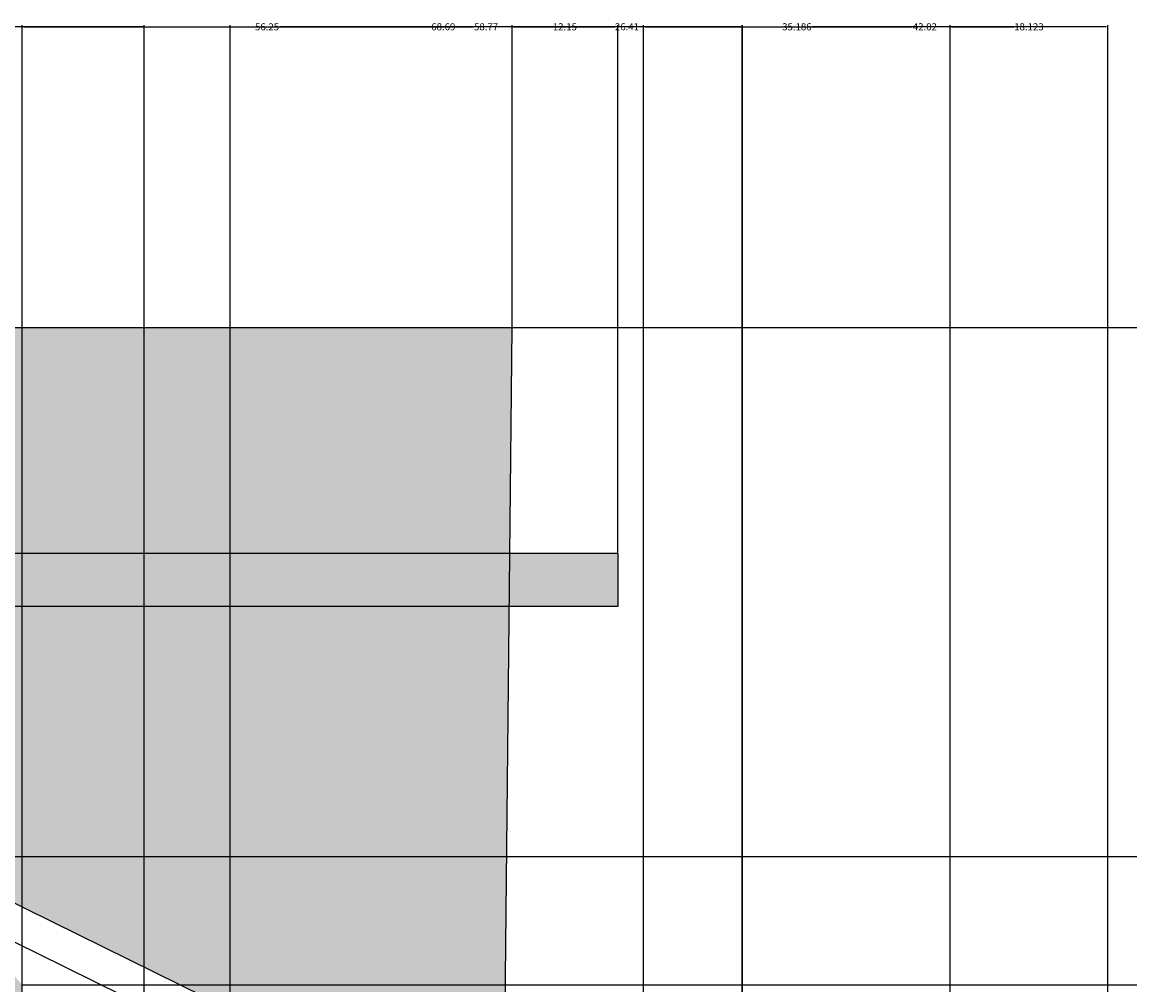
# Model space of a CAD drawing. Units: inches. Extents: x 36 to 594, y 79 to 831.
# Tile 28 of 30: x 342 to 469, y 721 to 831. Entities that reach past the tile are written whole.
import ezdxf

# ---------------------------------------------------------------- set-up
doc = ezdxf.new("R2010")
doc.units = ezdxf.units.IN
doc.header["$MEASUREMENT"] = 0
for name, color, linetype, lineweight in [('A-ANNO-DIMS', 2, 'Continuous', 18), ('A-ELEV', 7, 'Continuous', 25), ('A-ELEV-PATT', 8, 'Continuous', 13)]:
    doc.layers.add(name, color=color, linetype=linetype, lineweight=lineweight)
doc.styles.get("Standard").update_dxf_attribs({"font": 'arial.ttf'})
doc.dimstyles.get("Standard").update_dxf_attribs({"dimtxt": 0.8125, "dimasz": 0.18, "dimexe": 0.18, "dimexo": 0.0625, "dimgap": 0.09, "dimtad": 0, "dimtih": 1, "dimtoh": 1, "dimdec": 4, "dimzin": 0, "dimdsep": 46, "dimlunit": 4, "dimtxsty": 'Standard', "dimcen": 0.09, "dimadec": 0, "dimazin": 0, "dimtfac": 1, "dimtdec": 4, "dimtofl": 0, "dimtmove": 0, "dimatfit": 3, "dimfxl": 1, "dimtolj": 1, "dimtzin": 0, "dimarcsym": 0})

# ---------------------------------------------------------------- blocks, each defined once
blk = doc.blocks.new('*D16')
at = {"layer": 'A-ANNO-DIMS', "color": 0, "lineweight": -2, "transparency": 16777216}
for p, q in [((269.36, 796.11), (269.36, 830.73)), ((341.84, 720.66), (341.84, 830.73)), ((269.54, 830.55), (304.14, 830.55)), ((341.66, 830.55), (307.06, 830.55))]:
    blk.add_line(p, q, dxfattribs=at)
at = {"layer": 'A-ANNO-DIMS', "color": 0, "transparency": 16777216}
for points in [[(269.54, 830.58), (269.54, 830.52), (269.36, 830.55)], [(341.66, 830.58), (341.66, 830.52), (341.84, 830.55)]]:
    blk.add_solid(points, dxfattribs=at)
at = {"layer": 'Defpoints', "color": 0, "transparency": 16777216}
for p in [(341.84, 830.55), (269.36, 796.05), (341.84, 720.59)]:
    blk.add_point(p, dxfattribs=at)
at = {"layer": 'A-ANNO-DIMS', "color": 0, "transparency": 16777216, "insert": (305.6, 830.55), "char_height": 0.812, "attachment_point": 5}
blk.add_mtext('\\A1;72.48', dxfattribs=at)
blk = doc.blocks.new('*D17')
at = {"layer": 'A-ANNO-DIMS', "color": 0, "lineweight": -2, "transparency": 16777216}
for p, q in [((341.84, 720.66), (341.84, 830.73)), ((398.09, 796.11), (398.09, 830.73)), ((342.02, 830.55), (368.5, 830.55)), ((397.91, 830.55), (371.43, 830.55))]:
    blk.add_line(p, q, dxfattribs=at)
at = {"layer": 'A-ANNO-DIMS', "color": 0, "transparency": 16777216}
for points in [[(342.02, 830.58), (342.02, 830.52), (341.84, 830.55)], [(397.91, 830.58), (397.91, 830.52), (398.09, 830.55)]]:
    blk.add_solid(points, dxfattribs=at)
at = {"layer": 'Defpoints', "color": 0, "transparency": 16777216}
for p in [(398.09, 830.55), (398.09, 796.05), (341.84, 720.59)]:
    blk.add_point(p, dxfattribs=at)
at = {"layer": 'A-ANNO-DIMS', "color": 0, "transparency": 16777216, "insert": (369.96, 830.55), "char_height": 0.812, "attachment_point": 5}
blk.add_mtext('\\A1;56.25', dxfattribs=at)
blk = doc.blocks.new('*D18')
at = {"layer": 'A-ANNO-DIMS', "color": 0, "lineweight": -2, "transparency": 16777216}
for p, q in [((398.09, 796.11), (398.09, 830.73)), ((424.5, 594.27), (424.5, 830.73)), ((398.27, 830.55), (409.9, 830.55)), ((424.32, 830.55), (412.68, 830.55))]:
    blk.add_line(p, q, dxfattribs=at)
at = {"layer": 'A-ANNO-DIMS', "color": 0, "transparency": 16777216}
for points in [[(398.27, 830.58), (398.27, 830.52), (398.09, 830.55)], [(424.32, 830.58), (424.32, 830.52), (424.5, 830.55)]]:
    blk.add_solid(points, dxfattribs=at)
at = {"layer": 'Defpoints', "color": 0, "transparency": 16777216}
for p in [(424.5, 830.55), (398.09, 796.05), (424.5, 594.21)]:
    blk.add_point(p, dxfattribs=at)
at = {"layer": 'A-ANNO-DIMS', "color": 0, "transparency": 16777216, "insert": (411.29, 830.55), "char_height": 0.812, "attachment_point": 5}
blk.add_mtext('\\A1;26.41', dxfattribs=at)
blk = doc.blocks.new('*D19')
at = {"layer": 'A-ANNO-DIMS', "color": 0, "lineweight": -2, "transparency": 16777216}
for p, q in [((424.5, 594.27), (424.5, 830.73)), ((466.51, 668.28), (466.51, 830.73)), ((424.68, 830.55), (444.03, 830.55)), ((466.33, 830.55), (446.98, 830.55))]:
    blk.add_line(p, q, dxfattribs=at)
at = {"layer": 'A-ANNO-DIMS', "color": 0, "transparency": 16777216}
for points in [[(424.68, 830.58), (424.68, 830.52), (424.5, 830.55)], [(466.33, 830.58), (466.33, 830.52), (466.51, 830.55)]]:
    blk.add_solid(points, dxfattribs=at)
at = {"layer": 'Defpoints', "color": 0, "transparency": 16777216}
for p in [(466.51, 830.55), (466.51, 668.22), (424.5, 594.21)]:
    blk.add_point(p, dxfattribs=at)
at = {"layer": 'A-ANNO-DIMS', "color": 0, "transparency": 16777216, "insert": (445.5, 830.55), "char_height": 0.812, "attachment_point": 5}
blk.add_mtext('\\A1;42.02', dxfattribs=at)
blk = doc.blocks.new('*D20')
at = {"layer": 'A-ANNO-DIMS', "color": 0, "lineweight": -2, "transparency": 16777216}
for p, q in [((365.73, 594.27), (365.73, 830.73)), ((424.5, 594.27), (424.5, 830.73)), ((365.91, 830.55), (393.65, 830.55)), ((424.32, 830.55), (396.57, 830.55))]:
    blk.add_line(p, q, dxfattribs=at)
at = {"layer": 'A-ANNO-DIMS', "color": 0, "transparency": 16777216}
for points in [[(365.91, 830.58), (365.91, 830.52), (365.73, 830.55)], [(424.32, 830.58), (424.32, 830.52), (424.5, 830.55)]]:
    blk.add_solid(points, dxfattribs=at)
at = {"layer": 'Defpoints', "color": 0, "transparency": 16777216}
for p in [(424.5, 830.55), (365.73, 594.21), (424.5, 594.21)]:
    blk.add_point(p, dxfattribs=at)
at = {"layer": 'A-ANNO-DIMS', "color": 0, "transparency": 16777216, "insert": (395.11, 830.55), "char_height": 0.812, "attachment_point": 5}
blk.add_mtext('\\A1;58.77', dxfattribs=at)
blk = doc.blocks.new('*D23')
at = {"layer": 'A-ANNO-DIMS', "color": 0, "lineweight": -2, "transparency": 16777216}
for p, q in [((329.98, 735.4), (329.98, 830.73)), ((341.84, 720.66), (341.84, 830.73)), ((330.16, 830.55), (334.17, 830.55)), ((341.66, 830.55), (337.65, 830.55))]:
    blk.add_line(p, q, dxfattribs=at)
at = {"layer": 'A-ANNO-DIMS', "color": 0, "transparency": 16777216}
for points in [[(330.16, 830.58), (330.16, 830.52), (329.98, 830.55)], [(341.66, 830.58), (341.66, 830.52), (341.84, 830.55)]]:
    blk.add_solid(points, dxfattribs=at)
at = {"layer": 'Defpoints', "color": 0, "transparency": 16777216}
for p in [(341.84, 830.55), (329.98, 735.34), (341.84, 720.59)]:
    blk.add_point(p, dxfattribs=at)
at = {"layer": 'A-ANNO-DIMS', "color": 0, "transparency": 16777216, "insert": (335.91, 830.55), "char_height": 0.812, "attachment_point": 5}
blk.add_mtext('\\A1;11.855', dxfattribs=at)
blk = doc.blocks.new('*D24')
at = {"layer": 'A-ANNO-DIMS', "color": 0, "lineweight": -2, "transparency": 16777216}
for p, q in [((448.39, 668.27), (448.39, 830.73)), ((466.51, 668.28), (466.51, 830.73)), ((448.57, 830.55), (455.71, 830.55)), ((466.33, 830.55), (459.19, 830.55))]:
    blk.add_line(p, q, dxfattribs=at)
at = {"layer": 'A-ANNO-DIMS', "color": 0, "transparency": 16777216}
for points in [[(448.57, 830.58), (448.57, 830.52), (448.39, 830.55)], [(466.33, 830.58), (466.33, 830.52), (466.51, 830.55)]]:
    blk.add_solid(points, dxfattribs=at)
at = {"layer": 'Defpoints', "color": 0, "transparency": 16777216}
for p in [(466.51, 830.55), (448.39, 668.21), (466.51, 668.22)]:
    blk.add_point(p, dxfattribs=at)
at = {"layer": 'A-ANNO-DIMS', "color": 0, "transparency": 16777216, "insert": (457.45, 830.55), "char_height": 0.812, "attachment_point": 5}
blk.add_mtext('\\A1;18.123', dxfattribs=at)
blk = doc.blocks.new('*D26')
at = {"layer": 'A-ANNO-DIMS', "color": 0, "lineweight": -2, "transparency": 16777216}
for p, q in [((398.09, 796.11), (398.09, 830.73)), ((410.24, 770.21), (410.24, 830.73)), ((398.27, 830.55), (402.74, 830.55)), ((410.06, 830.55), (405.59, 830.55))]:
    blk.add_line(p, q, dxfattribs=at)
at = {"layer": 'A-ANNO-DIMS', "color": 0, "transparency": 16777216}
for points in [[(398.27, 830.58), (398.27, 830.52), (398.09, 830.55)], [(410.06, 830.58), (410.06, 830.52), (410.24, 830.55)]]:
    blk.add_solid(points, dxfattribs=at)
at = {"layer": 'Defpoints', "color": 0, "transparency": 16777216}
for p in [(410.24, 830.55), (398.09, 796.05), (410.24, 770.15)]:
    blk.add_point(p, dxfattribs=at)
at = {"layer": 'A-ANNO-DIMS', "color": 0, "transparency": 16777216, "insert": (404.16, 830.55), "char_height": 0.812, "attachment_point": 5}
blk.add_mtext('\\A1;12.15', dxfattribs=at)
blk = doc.blocks.new('*D37')
at = {"layer": 'A-ANNO-DIMS', "color": 0, "lineweight": -2, "transparency": 16777216}
for p, q in [((330.04, 735.34), (592.85, 735.34)), ((592.67, 735.16), (592.67, 702.28)), ((592.67, 668.39), (592.67, 701.27)), ((448.45, 668.21), (592.85, 668.21))]:
    blk.add_line(p, q, dxfattribs=at)
at = {"layer": 'A-ANNO-DIMS', "color": 0, "transparency": 16777216}
for points in [[(592.64, 735.16), (592.7, 735.16), (592.67, 735.34)], [(592.64, 668.39), (592.7, 668.39), (592.67, 668.21)]]:
    blk.add_solid(points, dxfattribs=at)
at = {"layer": 'Defpoints', "color": 0, "transparency": 16777216}
for p in [(329.98, 735.34), (592.67, 735.34), (448.39, 668.21)]:
    blk.add_point(p, dxfattribs=at)
at = {"layer": 'A-ANNO-DIMS', "color": 0, "transparency": 16777216, "insert": (592.67, 701.77), "char_height": 0.812, "attachment_point": 5}
blk.add_mtext('\\A1;67.12', dxfattribs=at)
blk = doc.blocks.new('*D38')
at = {"layer": 'A-ANNO-DIMS', "color": 0, "lineweight": -2, "transparency": 16777216}
for p, q in [((398.15, 796.05), (592.85, 796.05)), ((592.67, 795.87), (592.67, 766.2)), ((592.67, 735.52), (592.67, 765.19)), ((330.04, 735.34), (592.85, 735.34))]:
    blk.add_line(p, q, dxfattribs=at)
at = {"layer": 'A-ANNO-DIMS', "color": 0, "transparency": 16777216}
for points in [[(592.64, 795.87), (592.7, 795.87), (592.67, 796.05)], [(592.64, 735.52), (592.7, 735.52), (592.67, 735.34)]]:
    blk.add_solid(points, dxfattribs=at)
at = {"layer": 'Defpoints', "color": 0, "transparency": 16777216}
for p in [(398.09, 796.05), (592.67, 796.05), (329.98, 735.34)]:
    blk.add_point(p, dxfattribs=at)
at = {"layer": 'A-ANNO-DIMS', "color": 0, "transparency": 16777216, "insert": (592.67, 765.69), "char_height": 0.812, "attachment_point": 5}
blk.add_mtext('\\A1;60.71', dxfattribs=at)
blk = doc.blocks.new('*D39')
at = {"layer": 'A-ANNO-DIMS', "color": 0, "lineweight": -2, "transparency": 16777216}
for p, q in [((413.2, 653.92), (413.2, 830.73)), ((448.39, 668.27), (448.39, 830.73)), ((413.38, 830.55), (429.02, 830.55)), ((448.21, 830.55), (432.57, 830.55))]:
    blk.add_line(p, q, dxfattribs=at)
at = {"layer": 'A-ANNO-DIMS', "color": 0, "transparency": 16777216}
for points in [[(413.38, 830.58), (413.38, 830.52), (413.2, 830.55)], [(448.21, 830.58), (448.21, 830.52), (448.39, 830.55)]]:
    blk.add_solid(points, dxfattribs=at)
at = {"layer": 'Defpoints', "color": 0, "transparency": 16777216}
for p in [(448.39, 830.55), (448.39, 668.21), (413.2, 653.86)]:
    blk.add_point(p, dxfattribs=at)
at = {"layer": 'A-ANNO-DIMS', "color": 0, "transparency": 16777216, "insert": (430.8, 830.55), "char_height": 0.812, "attachment_point": 5}
blk.add_mtext('\\A1;35.186', dxfattribs=at)
blk = doc.blocks.new('*D41')
at = {"layer": 'A-ANNO-DIMS', "color": 0, "lineweight": -2, "transparency": 16777216}
for p, q in [((341.9, 720.59), (592.85, 720.59)), ((592.67, 720.41), (592.67, 694.91)), ((592.67, 668.39), (592.67, 693.9)), ((448.45, 668.21), (592.85, 668.21))]:
    blk.add_line(p, q, dxfattribs=at)
at = {"layer": 'A-ANNO-DIMS', "color": 0, "transparency": 16777216}
for points in [[(592.64, 720.41), (592.7, 720.41), (592.67, 720.59)], [(592.64, 668.39), (592.7, 668.39), (592.67, 668.21)]]:
    blk.add_solid(points, dxfattribs=at)
at = {"layer": 'Defpoints', "color": 0, "transparency": 16777216}
for p in [(341.84, 720.59), (592.67, 720.59), (448.39, 668.21)]:
    blk.add_point(p, dxfattribs=at)
at = {"layer": 'A-ANNO-DIMS', "color": 0, "transparency": 16777216, "insert": (592.67, 694.4), "char_height": 0.812, "attachment_point": 5}
blk.add_mtext('\\A1;52.38', dxfattribs=at)
blk = doc.blocks.new('*D59')
at = {"layer": 'A-ANNO-DIMS', "color": 0, "lineweight": -2, "transparency": 16777216}
for p, q in [((355.86, 355.15), (355.86, 830.73)), ((424.55, 355.15), (424.55, 830.73)), ((356.04, 830.55), (388.74, 830.55)), ((424.37, 830.55), (391.67, 830.55))]:
    blk.add_line(p, q, dxfattribs=at)
at = {"layer": 'A-ANNO-DIMS', "color": 0, "transparency": 16777216}
for points in [[(356.04, 830.58), (356.04, 830.52), (355.86, 830.55)], [(424.37, 830.58), (424.37, 830.52), (424.55, 830.55)]]:
    blk.add_solid(points, dxfattribs=at)
at = {"layer": 'Defpoints', "color": 0, "transparency": 16777216}
for p in [(424.55, 830.55), (355.86, 355.08), (424.55, 355.08)]:
    blk.add_point(p, dxfattribs=at)
at = {"layer": 'A-ANNO-DIMS', "color": 0, "transparency": 16777216, "insert": (390.2, 830.55), "char_height": 0.812, "attachment_point": 5}
blk.add_mtext('\\A1;68.69', dxfattribs=at)
blk = doc.blocks.new('*D95')
at = {"layer": 'A-ANNO-DIMS', "color": 0, "lineweight": -2, "transparency": 16777216}
for p, q in [((260.51, 524.67), (260.51, 830.73)), ((341.84, 524.67), (341.84, 830.73)), ((260.69, 830.55), (299.71, 830.55)), ((341.66, 830.55), (302.63, 830.55))]:
    blk.add_line(p, q, dxfattribs=at)
at = {"layer": 'A-ANNO-DIMS', "color": 0, "transparency": 16777216}
for points in [[(260.69, 830.58), (260.69, 830.52), (260.51, 830.55)], [(341.66, 830.58), (341.66, 830.52), (341.84, 830.55)]]:
    blk.add_solid(points, dxfattribs=at)
at = {"layer": 'Defpoints', "color": 0, "transparency": 16777216}
for p in [(341.84, 830.55), (260.51, 524.6), (341.84, 524.6)]:
    blk.add_point(p, dxfattribs=at)
at = {"layer": 'A-ANNO-DIMS', "color": 0, "transparency": 16777216, "insert": (301.17, 830.55), "char_height": 0.812, "attachment_point": 5}
blk.add_mtext('\\A1;81.33', dxfattribs=at)
blk = doc.blocks.new('*D107')
at = {"layer": 'A-ANNO-DIMS', "color": 0, "lineweight": -2, "transparency": 16777216}
for p, q in [((269.04, 404.34), (269.04, 830.73)), ((355.86, 404.34), (355.86, 830.73)), ((269.22, 830.55), (310.99, 830.55)), ((355.68, 830.55), (313.91, 830.55))]:
    blk.add_line(p, q, dxfattribs=at)
at = {"layer": 'A-ANNO-DIMS', "color": 0, "transparency": 16777216}
for points in [[(269.22, 830.58), (269.22, 830.52), (269.04, 830.55)], [(355.68, 830.58), (355.68, 830.52), (355.86, 830.55)]]:
    blk.add_solid(points, dxfattribs=at)
at = {"layer": 'Defpoints', "color": 0, "transparency": 16777216}
for p in [(355.86, 830.55), (269.04, 404.27), (355.86, 404.27)]:
    blk.add_point(p, dxfattribs=at)
at = {"layer": 'A-ANNO-DIMS', "color": 0, "transparency": 16777216, "insert": (312.45, 830.55), "char_height": 0.812, "attachment_point": 5}
blk.add_mtext('\\A1;86.82', dxfattribs=at)
blk = doc.blocks.new('*D129')
at = {"layer": 'A-ANNO-DIMS', "color": 0, "lineweight": -2, "transparency": 16777216}
for p, q in [((316.05, 630.1), (316.05, 830.73)), ((341.84, 630.1), (341.84, 830.73)), ((316.23, 830.55), (327.16, 830.55)), ((341.66, 830.55), (330.73, 830.55))]:
    blk.add_line(p, q, dxfattribs=at)
at = {"layer": 'A-ANNO-DIMS', "color": 0, "transparency": 16777216}
for points in [[(316.23, 830.58), (316.23, 830.52), (316.05, 830.55)], [(341.66, 830.58), (341.66, 830.52), (341.84, 830.55)]]:
    blk.add_solid(points, dxfattribs=at)
at = {"layer": 'Defpoints', "color": 0, "transparency": 16777216}
for p in [(341.84, 830.55), (316.05, 630.04), (341.84, 630.04)]:
    blk.add_point(p, dxfattribs=at)
at = {"layer": 'A-ANNO-DIMS', "color": 0, "transparency": 16777216, "insert": (328.94, 830.55), "char_height": 0.812, "attachment_point": 5}
blk.add_mtext('\\A1;25.785', dxfattribs=at)

msp = doc.modelspace()

# ---------------------------------------------------------------- hatches: boundary and pattern name
at = {"layer": 'A-ELEV-PATT'}
h = msp.add_hatch(color=256, dxfattribs=at)
h.dxf.hatch_style = 1
h.paths.add_polyline_path([(398.0873, 796.0465), (269.3592, 796.0465), (269.3592, 770.1455), (397.8159, 770.1455)])
h.paths.add_polyline_path([(397.7518, 764.0341), (269.3592, 764.0341), (269.3592, 630.0394), (341.8367, 630.0394), (341.8367, 720.595), (335.0881, 728.3699), (329.982, 735.3373), (345.3661, 727.7743), (397.1052, 702.3389)])
h.paths.add_polyline_path([(341.8367, 594.2124), (201.4189, 594.2124), (201.4189, 475.4136), (232.8216, 475.4136), (232.8216, 524.6037), (341.8367, 524.6037)])
h.paths.add_polyline_path([(177.525, 594.2124), (118.7598, 594.2124), (118.7598, 450.2124), (177.525, 450.2124)])
h.paths.add_polyline_path([(424.4958, 594.2124), (365.7306, 594.2124), (365.7306, 450.2124), (424.4958, 450.2124)])
h.paths.add_polyline_path([(241.3553, 404.2737), (355.8569, 404.2737), (355.8569, 355.0836), (424.5492, 355.0836), (424.5492, 425.7333), (118.7598, 426.2844), (118.7598, 355.0836), (241.3553, 355.0836)])
h.paths.add_polyline_path([(448.3898, 306.2124), (217.0273, 306.2124), (217.0273, 142.2124), (254.0293, 142.2124), (254.0293, 150.9347), (254.0293, 286.1802), (401.5491, 286.1802), (401.5491, 150.9347), (401.5491, 142.2124), (448.3898, 142.2124)])
h.paths.add_polyline_path([(448.3898, 142.2124), (401.5491, 142.2124), (217.0273, 142.2124), (217.0273, 114.2124), (448.3898, 114.2124)])
h.paths.add_polyline_path([(217.0273, 306.2124), (174.7353, 306.2124), (94.8658, 306.2124), (94.8658, 162.2124), (103.3368, 162.2124), (103.3368, 264.6224), (103.3368, 286.1802), (217.0273, 286.1802)])
h = msp.add_hatch(color=256, dxfattribs=at)
h.dxf.hatch_style = 1
h.paths.add_polyline_path([(94.8658, 608.6081), (72.1733, 608.6081), (72.1733, 603.598), (94.8658, 603.598)])
h.paths.add_polyline_path([(94.8658, 427.5982), (72.1733, 427.5982), (72.1733, 422.5882), (94.8658, 422.5882)])
h.paths.add_polyline_path([(94.8658, 299.486), (72.1733, 299.486), (72.1733, 294.4759), (94.8658, 294.4759)])
h.paths.add_polyline_path([(269.3592, 770.1455), (260.5727, 770.1455), (260.5727, 764.0341), (269.3592, 764.0341)])
h.paths.add_polyline_path([(410.2381, 770.1455), (269.3592, 770.1455), (269.3592, 764.0341), (410.2381, 764.0341)])

# ---------------------------------------------------------------- linework, layer by layer
at = {"layer": 'A-ELEV'}
for p, q in [((269.3592, 796.0465), (398.0873, 796.0465)), ((398.0873, 796.0465), (397.1052, 702.3389)), ((345.3661, 727.7743), (329.982, 735.3373)), ((343.6014, 724.1846), (335.0881, 728.3699)), ((451.9192, 675.3917), (345.3661, 727.7743)), ((450.1545, 671.802), (343.6014, 724.1846))]:
    msp.add_line(p, q, dxfattribs=at)
msp.add_lwpolyline([(260.5727, 770.1455), (410.2381, 770.1455), (410.2381, 764.0341), (260.5727, 764.0341)], close=True, dxfattribs=at)

# ---------------------------------------------------------------- dimensions: what is measured, and where the dimension line sits
at = {"layer": 'A-ANNO-DIMS'}
for base, p1, p2, override, picture, middle in [((341.8367, 830.5465), (260.5056, 524.6037), (341.8367, 524.6037), {"dimdec": 2, "dimlfac": 1, "dimrnd": 0, "dimzin": 0, "dimdsep": 46, "dimlunit": 2}, '*D95', (301.1711, 830.5465)), ((355.8569, 830.5465), (269.0393, 404.2737), (355.8569, 404.2737), {"dimdec": 2, "dimlfac": 1, "dimrnd": 0, "dimzin": 0, "dimdsep": 46, "dimlunit": 2}, '*D107', (312.4481, 830.5465)), ((341.8367, 830.5465), (269.3592, 796.0465), (341.8367, 720.595), {"dimdec": 2, "dimlfac": 1, "dimrnd": 0, "dimzin": 0, "dimdsep": 46, "dimlunit": 2}, '*D16', (305.5979, 830.5465)), ((341.8367, 830.5465), (316.0513, 630.0394), (341.8367, 630.0394), {"dimdec": 3, "dimlfac": 1, "dimrnd": 0, "dimzin": 0, "dimdsep": 46, "dimlunit": 2}, '*D129', (328.944, 830.5465)), ((341.8367, 830.5465), (329.982, 735.3373), (341.8367, 720.595), {"dimdec": 3, "dimlfac": 1, "dimrnd": 0, "dimzin": 0, "dimdsep": 46, "dimlunit": 2}, '*D23', (335.9093, 830.5465)), ((398.0873, 830.5465), (341.8367, 720.595), (398.0873, 796.0465), {"dimdec": 2, "dimlfac": 1, "dimrnd": 0, "dimzin": 0, "dimdsep": 46, "dimlunit": 2}, '*D17', (369.962, 830.5465)), ((424.5492, 830.5465), (355.8569, 355.0836), (424.5492, 355.0836), {"dimdec": 2, "dimlfac": 1, "dimrnd": 0, "dimzin": 0, "dimdsep": 46, "dimlunit": 2}, '*D59', (390.203, 830.5465)), ((424.4958, 830.5465), (365.7306, 594.2124), (424.4958, 594.2124), {"dimdec": 2, "dimlfac": 1, "dimrnd": 0, "dimzin": 0, "dimdsep": 46, "dimlunit": 2}, '*D20', (395.1132, 830.5465)), ((424.4958, 830.5465), (398.0873, 796.0465), (424.4958, 594.2124), {"dimdec": 2, "dimlfac": 1, "dimrnd": 0, "dimzin": 0, "dimdsep": 46, "dimlunit": 2}, '*D18', (411.2916, 830.5465)), ((410.2381, 830.5465), (398.0873, 796.0465), (410.2381, 770.1455), {"dimdec": 2, "dimlfac": 1, "dimrnd": 0, "dimzin": 0, "dimdsep": 46, "dimlunit": 2}, '*D26', (404.1627, 830.5465)), ((448.38977, 830.54647), (413.2033, 653.85634), (448.38977, 668.21236), {"dimdec": 3, "dimlfac": 1, "dimrnd": 0, "dimzin": 0, "dimdsep": 46, "dimlunit": 2}, '*D39', (430.79654, 830.54647)), ((466.5128, 830.5465), (424.4958, 594.2124), (466.5128, 668.2174), {"dimdec": 2, "dimlfac": 1, "dimrnd": 0, "dimzin": 0, "dimdsep": 46, "dimlunit": 2}, '*D19', (445.5043, 830.5465)), ((466.5128, 830.5465), (448.3898, 668.2124), (466.5128, 668.2174), {"dimdec": 3, "dimlfac": 1, "dimrnd": 0, "dimzin": 0, "dimdsep": 46, "dimlunit": 2}, '*D24', (457.4513, 830.5465))]:
    dim = msp.add_linear_dim(base=base, p1=p1, p2=p2, dimstyle='Standard', override=override, dxfattribs=at)
    dim.commit()
    dim.dimension.update_dxf_attribs({"geometry": picture, "text_midpoint": middle})
for base, p1, p2, picture, middle in [((592.6689, 796.0465), (329.982, 735.3373), (398.0873, 796.0465), '*D38', (592.6689, 765.6919)), ((592.6689, 735.3373), (448.3898, 668.2124), (329.982, 735.3373), '*D37', (592.6689, 701.7748)), ((592.6689, 720.595), (448.3898, 668.2124), (341.8367, 720.595), '*D41', (592.6689, 694.4037))]:
    dim = msp.add_linear_dim(base=base, p1=p1, p2=p2, angle=90, dimstyle='Standard', override={"dimdec": 2, "dimlfac": 1, "dimrnd": 0, "dimzin": 0, "dimdsep": 46, "dimlunit": 2}, dxfattribs=at)
    dim.commit()
    dim.dimension.update_dxf_attribs({"geometry": picture, "text_midpoint": middle})

doc.saveas('drawing.dxf')
